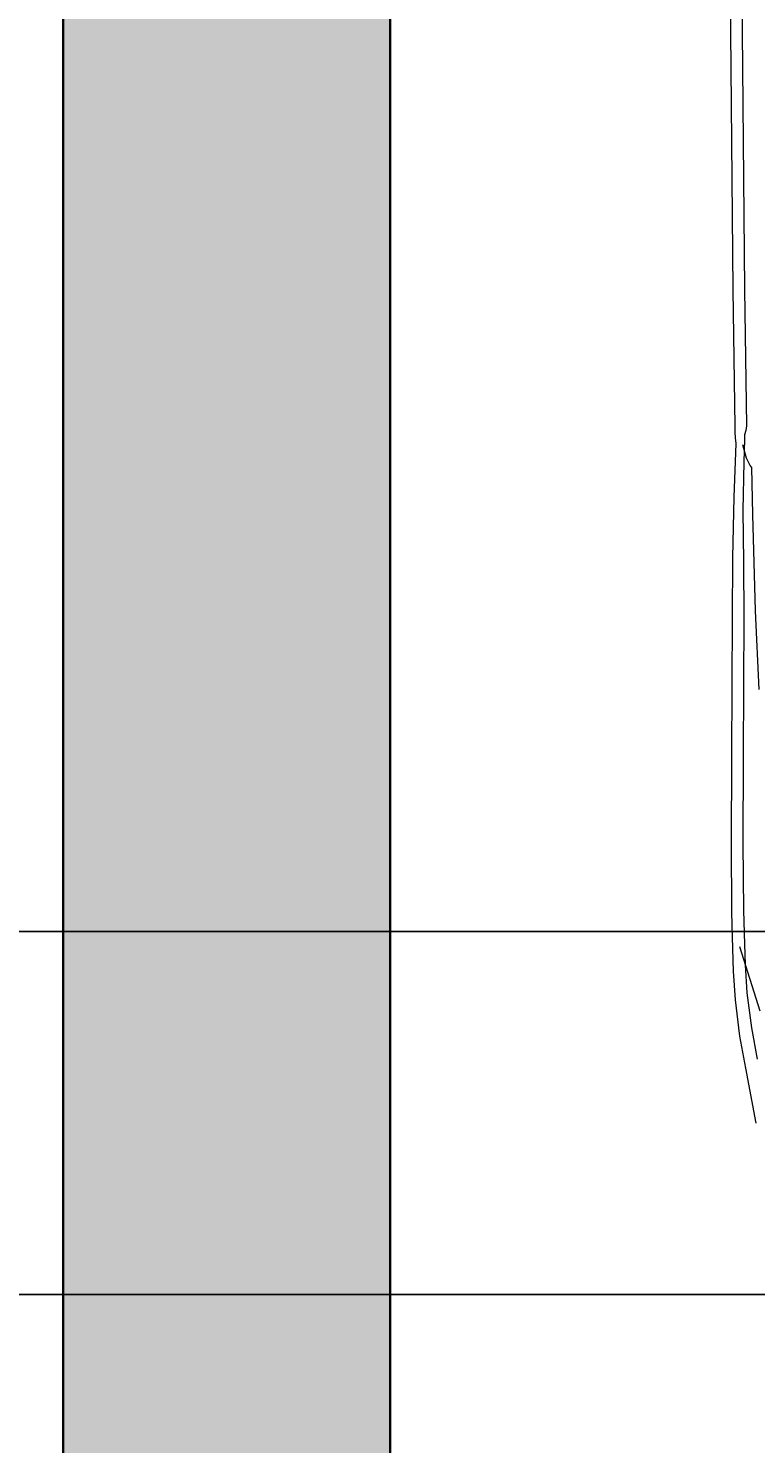
# Model space of a CAD drawing. Units: inches. Extents: x -5 to 482, y -460 to 66.
# Tile 3 of 31: x 32 to 52, y -390 to -351. Entities that reach past the tile are written whole.
import ezdxf

# ---------------------------------------------------------------- set-up
doc = ezdxf.new("R2010")
doc.units = ezdxf.units.IN
doc.header["$MEASUREMENT"] = 0
for name, color, linetype, lineweight in [('A-ANNO-DIMS', 2, 'Continuous', 18), ('A-EQPM-VEHI', 8, 'Continuous', 13), ('A-WALL', 7, 'Continuous', 35), ('A-WALL-PATT', 152, 'Continuous', 13)]:
    doc.layers.add(name, color=color, linetype=linetype, lineweight=lineweight)
doc.styles.get("Standard").update_dxf_attribs({"font": 'arial.ttf'})
doc.dimstyles.get("Standard").update_dxf_attribs({"dimtxt": 0.18, "dimasz": 0.18, "dimexe": 0.18, "dimexo": 0.0625, "dimgap": 0.09, "dimtad": 0, "dimtih": 1, "dimtoh": 1, "dimdec": 0, "dimzin": 0, "dimdsep": 46, "dimlunit": 3, "dimtxsty": 'Standard', "dimcen": 0.09, "dimadec": 0, "dimazin": 0, "dimtfac": 1, "dimtdec": 0, "dimtofl": 0, "dimtmove": 0, "dimatfit": 3, "dimfxl": 1, "dimtolj": 1, "dimtzin": 0, "dimarcsym": 0})

# ---------------------------------------------------------------- blocks, each defined once
blk = doc.blocks.new('*D72')
at = {"layer": 'A-ANNO-DIMS', "color": 0, "lineweight": -2, "transparency": 16777216}
for p, q in [((144.314, -375.861), (-4.903, -375.861)), ((-4.723, -376.041), (-4.723, -380.679)), ((-4.723, -385.681), (-4.723, -381.043)), ((144.314, -385.861), (-4.903, -385.861))]:
    blk.add_line(p, q, dxfattribs=at)
at = {"layer": 'A-ANNO-DIMS', "color": 0, "transparency": 16777216}
for points in [[(-4.753, -376.041), (-4.693, -376.041), (-4.723, -375.861)], [(-4.753, -385.681), (-4.693, -385.681), (-4.723, -385.861)]]:
    blk.add_solid(points, dxfattribs=at)
at = {"layer": 'Defpoints', "color": 0, "transparency": 16777216}
for p in [(144.377, -375.861), (-4.723, -385.861), (144.377, -385.861)]:
    blk.add_point(p, dxfattribs=at)
at = {"layer": 'A-ANNO-DIMS', "color": 0, "transparency": 16777216, "insert": (-4.723, -380.861), "char_height": 0.18, "attachment_point": 5}
blk.add_mtext('\\A1;0\'-10"', dxfattribs=at)

msp = doc.modelspace()

# ---------------------------------------------------------------- hatches: boundary and pattern name
at = {"layer": 'A-WALL-PATT'}
h = msp.add_hatch(color=256, dxfattribs=at)
h.dxf.hatch_style = 1
h.paths.add_polyline_path([(149.377, -412.849), (144.377, -412.849), (144.377, -283.849), (144.377, -279.349), (133.877, -279.349), (133.877, -283.849), (139.877, -283.849), (139.877, -412.849), (133.51, -412.849), (133.51, -413.916), (102.652, -413.916), (102.652, -421.02), (133.51, -421.02), (133.51, -421.849), (149.377, -421.849)])
h.paths.add_polyline_path([(226.054, -412.849), (218.877, -412.849), (218.877, -350.849), (262.877, -350.849), (262.877, -386.849), (267.377, -386.849), (267.377, -283.849), (270.377, -283.849), (270.377, -279.349), (244.877, -279.349), (244.877, -283.849), (262.877, -283.849), (262.877, -346.349), (218.877, -346.349), (218.877, -283.849), (220.877, -283.849), (220.877, -279.349), (214.377, -279.349), (214.377, -283.849), (214.377, -412.849), (209.377, -412.849), (209.377, -421.849), (226.054, -421.849)])
h.paths.add_polyline_path([(315.815, -412.849), (250.054, -412.849), (250.054, -421.849), (315.815, -421.849)])
h.paths.add_polyline_path([(430.377, -378.349), (421.377, -378.349), (421.377, -412.849), (375.815, -412.849), (375.815, -421.849), (430.377, -421.849)])
h.paths.add_polyline_path([(78.691, -413.916), (47.68, -413.916), (47.68, -412.849), (41.877, -412.849), (41.877, -283.849), (109.877, -283.849), (109.877, -279.349), (41.877, -279.349), (41.877, -241.849), (32.877, -241.849), (32.877, -421.849), (47.68, -421.849), (47.68, -421.02), (78.691, -421.02)])
h.paths.add_polyline_path([(41.877, -144.349), (154.377, -144.349), (154.377, -137.849), (149.877, -137.849), (149.877, -139.849), (41.877, -139.849), (41.877, -97.849), (32.877, -97.849), (32.877, -181.849), (41.877, -181.849)])
h.paths.add_polyline_path([(430.377, -241.849), (421.377, -241.849), (421.377, -279.349), (309.377, -279.349), (309.377, -170.349), (304.877, -170.349), (304.877, -279.349), (294.377, -279.349), (294.377, -283.849), (421.377, -283.849), (421.377, -318.349), (430.377, -318.349)])
h.paths.add_polyline_path([(430.377, -119.849), (421.377, -119.849), (421.377, -139.849), (419.377, -139.849), (419.377, -144.349), (421.377, -144.349), (421.377, -181.849), (430.377, -181.849)])
h.paths.add_polyline_path([(395.377, -139.849), (377.377, -139.849), (377.377, -75.849), (421.377, -75.849), (421.377, -95.849), (430.377, -95.849), (430.377, -45.599), (421.377, -45.599), (421.377, -71.349), (377.377, -71.349), (377.377, -22.849), (372.877, -22.849), (372.877, -139.849), (242.877, -139.849), (242.877, -137.849), (238.377, -137.849), (238.377, -144.349), (304.877, -144.349), (304.877, -146.349), (309.377, -146.349), (309.377, -144.349), (395.377, -144.349)])
h.paths.add_polyline_path([(65.877, 13.151), (32.877, 13.151), (32.877, -37.849), (41.877, -37.849), (41.877, 4.151), (65.877, 4.151)])
h.paths.add_polyline_path([(166.377, 13.151), (125.877, 13.151), (125.877, 4.151), (149.877, 4.151), (149.877, -113.849), (154.377, -113.849), (154.377, 4.151), (166.377, 4.151)])
h.paths.add_polyline_path([(277.877, 13.151), (226.377, 13.151), (226.377, 4.151), (238.377, 4.151), (238.377, -113.849), (242.877, -113.849), (242.877, 4.151), (277.877, 4.151)])
h.paths.add_polyline_path([(430.377, 13.151), (337.877, 13.151), (337.877, 4.151), (372.877, 4.151), (372.877, 1.151), (377.377, 1.151), (377.377, 4.151), (421.377, 4.151), (421.377, -21.599), (430.377, -21.599)])

# ---------------------------------------------------------------- linework, layer by layer
at = {"layer": 'A-EQPM-VEHI'}
for p, q in [((51.274, -352.085), (51.247, -348.881)), ((51.559, -348.88), (51.586, -352.081)), ((51.331, -358.195), (51.274, -352.085)), ((51.586, -352.081), (51.643, -358.186)), ((51.381, -361.958), (51.331, -358.195)), ((51.643, -358.186), (51.693, -361.946)), ((51.386, -362.117), (51.381, -361.958)), ((51.693, -361.946), (51.675, -362.076)), ((51.393, -362.276), (51.386, -362.117)), ((51.413, -362.434), (51.393, -362.276)), ((51.636, -362.321), (51.623, -362.932)), ((51.639, -362.191), (51.636, -362.321)), ((51.675, -362.076), (51.639, -362.191)), ((51.357, -363.903), (51.413, -362.434)), ((51.698, -362.83), (51.595, -362.465)), ((51.623, -362.932), (51.594, -364.27)), ((51.796, -363.032), (51.698, -362.83)), ((51.839, -363.094), (51.796, -363.032)), ((51.869, -364.388), (51.839, -363.094)), ((51.323, -365.564), (51.357, -363.903)), ((51.594, -364.27), (51.609, -365.691)), ((51.944, -367.039), (51.869, -364.388)), ((51.312, -367.254), (51.323, -365.564)), ((51.609, -365.691), (51.624, -367.254)), ((52.041, -369.206), (51.944, -367.039)), ((51.303, -369.037), (51.312, -367.254)), ((51.624, -367.254), (51.616, -369.037)), ((51.287, -371.09), (51.303, -369.037)), ((51.616, -369.037), (51.599, -371.09)), ((51.278, -373.437), (51.287, -371.09)), ((51.599, -371.09), (51.59, -373.437)), ((51.294, -375.332), (51.278, -373.437)), ((51.59, -373.437), (51.608, -375.287)), ((51.322, -376.342), (51.294, -375.332)), ((51.608, -375.287), (51.64, -376.214)), ((51.337, -376.954), (51.322, -376.342)), ((51.502, -376.274), (52.059, -378.05)), ((51.64, -376.214), (51.658, -376.781)), ((51.658, -376.781), (51.707, -377.549)), ((51.388, -377.748), (51.337, -376.954)), ((51.707, -377.549), (51.831, -378.52)), ((51.514, -378.744), (51.388, -377.748)), ((51.679, -379.625), (51.514, -378.744)), ((51.831, -378.52), (51.992, -379.38)), ((51.962, -381.14), (51.679, -379.625))]:
    msp.add_line(p, q, dxfattribs=at)
at = {"layer": 'A-WALL'}
for p, q in [((32.877, 13.151), (32.877, -421.849)), ((41.877, -283.849), (41.877, -412.849))]:
    msp.add_line(p, q, dxfattribs=at)

# ---------------------------------------------------------------- dimensions: what is measured, and where the dimension line sits
at = {"layer": 'A-ANNO-DIMS'}
dim = msp.add_linear_dim(base=(-4.723, -385.861), p1=(144.377, -375.861), p2=(144.377, -385.861), angle=90, dimstyle='Standard', override={"dimdec": 1, "dimlfac": 1, "dimrnd": 0, "dimzin": 1, "dimdsep": 46, "dimlunit": 4, "dimfrac": 2}, dxfattribs=at)
dim.commit()
dim.dimension.update_dxf_attribs({"geometry": '*D72', "text_midpoint": (-4.723, -380.861)})

doc.saveas('drawing.dxf')
